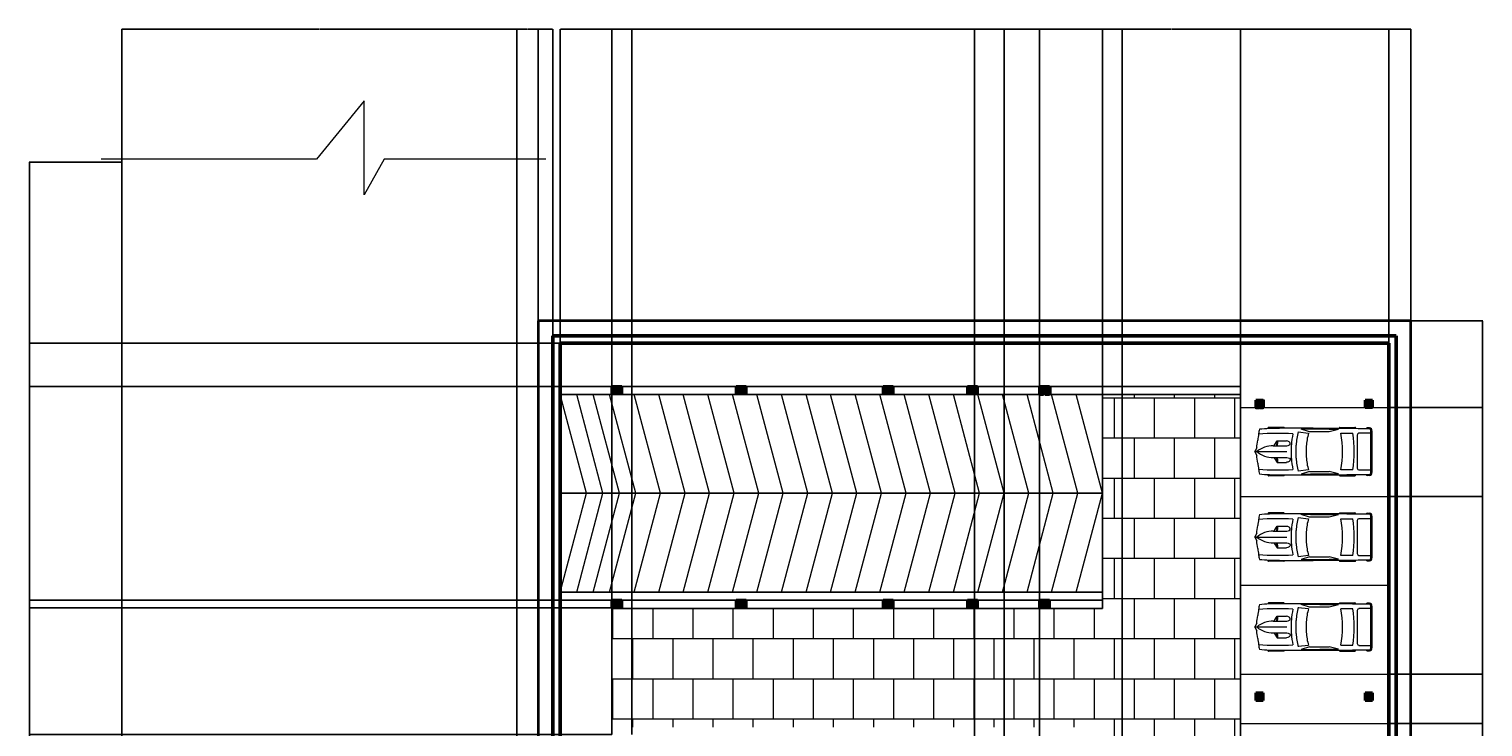
# Model space of a CAD drawing. Units: inches. Extents: x 154617 to 156384, y 250671 to 252576.
# Tile 6 of 6: x 154617 to 156384, y 251728 to 252576. Entities that reach past the tile are written whole.
import ezdxf

# ---------------------------------------------------------------- set-up
doc = ezdxf.new("R2010")
doc.units = ezdxf.units.IN
for name, color, linetype, lineweight in [('A-ANNO-DIMS', 2, 'Continuous', 18), ('A-EQPM-VEHI', 9, 'Continuous', 13), ('A-FLOR-DRIV', 5, 'Continuous', 25), ('A-FLOR-PATT', 112, 'Continuous', 13), ('A-FLOR-PRKG', 4, 'Continuous', 18), ('A-FLOR-RAMP', 7, 'Continuous', 25), ('A-FLOR-RAMP-PATT', 9, 'Continuous', 13), ('C-ANNO-BRKL', 7, 'Continuous', 18), ('C-PROP', 5, 'Continuous', 35), ('C-ROAD', 7, 'Continuous', 25), ('pillars', 6, 'Continuous', 40), ('walls', 4, 'Continuous', 50)]:
    doc.layers.add(name, color=color, linetype=linetype, lineweight=lineweight)
doc.styles.get("Standard").update_dxf_attribs({"font": 'arial.ttf'})
doc.dimstyles.get("Standard").update_dxf_attribs({"dimtxt": 0.18, "dimasz": 0.18, "dimexe": 0.18, "dimexo": 0.0625, "dimgap": 0.09, "dimtad": 0, "dimtih": 1, "dimtoh": 1, "dimdec": 4, "dimzin": 0, "dimdsep": 46, "dimtxsty": 'Standard', "dimcen": 0.09, "dimadec": 0, "dimazin": 0, "dimtfac": 1, "dimtdec": 4, "dimtofl": 0, "dimtmove": 0, "dimatfit": 3, "dimfxl": 1, "dimtolj": 1, "dimtzin": 0, "dimarcsym": 0})

# ---------------------------------------------------------------- blocks, each defined once
blk = doc.blocks.new('*U2')
for p, q in [((21.1, 37.4), (21.1, 36.8)), ((46.6, 38.9), (22.4, 38.9)), ((47.8, 37.4), (47.8, 37.4)), ((70, 31.5), (86.4, 29.4)), ((88, 31.9), (74.8, 35.9)), ((134.3, 35.6), (119.3, 31.8)), ((135.5, 37.1), (135.5, 37.4)), ((136.7, 38.9), (160.9, 38.9)), ((138.4, 29.4), (157.2, 29.4)), ((162.1, 37.4), (162.1, 36.8)), ((164.5, 26.4), (164.5, -26.4)), ((186.5, 29.4), (167, 29.4)), ((186.5, -33.5), (186.5, 33.5)), ((188.4, -32.8), (188.4, 32.8)), ((3.3, 6.1), (0.1, 0.4)), ((29.8, 9.5), (51.7, 9.5)), ((32.1, 9.5), (32.1, 11.2)), ((32.3, 11.6), (36.1, 17.2)), ((36.1, 17.2), (50.9, 17.2)), ((58.9, -10.8), (58.9, 10.8)), ((66.6, -10.5), (66.6, 10.5)), ((82.7, 8.5), (82.7, -8.5)), ((186.5, -10.5), (186.5, 10.5)), ((0, 0), (51.7, 0)), ((0.1, -0.4), (3.3, -6.1)), ((29.8, -9.5), (51.7, -9.5)), ((32.1, -9.5), (32.1, -11.2)), ((32.3, -11.6), (36.1, -17.2)), ((36.1, -17.2), (50.9, -17.2)), ((21.1, -37.4), (21.1, -36.8)), ((46.6, -38.9), (22.4, -38.9)), ((47.8, -37.4), (47.8, -37.4)), ((86.4, -29.4), (70, -31.5)), ((88, -31.9), (74.8, -35.9)), ((134.3, -35.6), (119.3, -31.8)), ((135.5, -37.1), (135.5, -37.4)), ((136.7, -38.9), (160.9, -38.9)), ((157.2, -29.4), (138.4, -29.4)), ((162.1, -37.4), (162.1, -36.8)), ((167, -29.4), (186.5, -29.4))]:
    blk.add_line(p, q)
for centre, major_axis, ratio, start_param, end_param in [((259.2, -27.5), (0, -305.3), 0.842304, 4.528606, 4.561838), ((266, -27.5), (0, 313.3), 0.842304, 1.367076, 1.39176), ((37.5, -594), (0, -623.3), 0.842304, 3.096046, 3.200911), ((41.2, -490.9), (0, 528.2), 0.842304, 0.00281, 0.075598), ((22.4, 37.4), (0, -1.48), 0.842304, 3.141593, 4.712389), ((64.5, -10555.6), (0, 10593), 0.842304, -0.013397, 0.002797), ((46.6, 37.4), (0, 1.48), 0.842304, -1.570796, 0), ((134.4, 5.4), (0, -89.8), 0.842304, 4.449482, 4.652344), ((135.3, 5.4), (0, 81.8), 0.842304, 1.245306, 1.50788), ((64.5, -10555.6), (0, -10591.5), 0.842304, 3.133765, 3.140441), ((149.6, 2.8), (0, -79.6), 0.842304, 4.372215, 4.640744), ((95.8, -3666.4), (0, -3698.2), 0.842304, 3.134049, 3.144098), ((136.7, 37.4), (0, -1.48), 0.842304, 3.141593, 4.712389), ((17.1, 0), (0, 147), 0.842304, 4.511394, 4.913384), ((35.9, 0), (0, 147), 0.842304, 4.511394, 4.913384), ((160.9, 37.4), (0, 1.48), 0.842304, -1.570796, 0), ((167, 26.4), (0, 2.96), 0.842304, 0, 1.570796), ((180.6, 35.8), (0, 2.22), 0.842304, -0.013017, 1.249894), ((64.5, -10556.4), (0, 10595.3), 0.842304, -0.013397, -0.013017), ((184, 32.8), (0, -5.25), 0.842304, 1.570796, 3.128196), ((184, 33.5), (0, -2.96), 0.842304, 1.570796, 3.128196), ((0.6, 0), (0, -0.74), 0.842304, 4.131459, 5.293319), ((-204.5, 52.4), (0, -251), 0.842304, 1.385369, 1.434372), ((29.8, -46.7), (0, 56.2), 0.842304, 0, 0.590319), ((32.7, 11.2), (0, 0.74), 0.842304, 0.879714, 1.570796), ((13, 17), (0, 27.4), 0.842304, 4.435146, 4.718221), ((14.2, 17), (0, 27.4), 0.842304, 4.435146, 4.718221), ((50.8, 13.3), (6.34, -0.36), 0.603834, -1.395552, 1.581315), ((-204.5, -52.4), (0, 251), 0.842304, -1.434372, -1.385369), ((29.8, 46.7), (0, 56.2), 0.842304, 2.551274, 3.141593), ((259.2, 27.5), (0, 305.3), 0.842304, 1.721348, 1.754579), ((32.7, -11.2), (0, -0.74), 0.842304, 4.712389, 5.403472), ((13, -17), (0, -27.4), 0.842304, 1.564964, 1.848039), ((14.2, -17), (0, -27.4), 0.842304, 1.564964, 1.848039), ((134.4, -5.4), (0, -89.8), 0.842304, -1.510751, -1.307889), ((135.3, -5.4), (0, -81.8), 0.842304, -1.50788, -1.245306), ((149.6, -2.8), (0, -79.6), 0.842304, -1.499151, -1.230623), ((266, 27.5), (0, 313.3), 0.842304, 1.749832, 1.774517), ((37.5, 594), (0, -623.3), 0.842304, -0.059319, 0.045547), ((41.2, 490.9), (0, -528.2), 0.842304, -0.075598, -0.00281), ((22.4, -37.4), (0, 1.48), 0.842304, 1.570796, 3.141593), ((64.5, 10555.6), (0, 10593), 0.842304, 3.138796, 3.15499), ((46.6, -37.4), (0, -1.48), 0.842304, 0, 1.570796), ((64.5, 10555.6), (0, -10591.5), 0.842304, 0.001152, 0.007828), ((95.8, 3666.4), (0, -3698.2), 0.842304, -0.002505, 0.007544), ((136.7, -37.4), (0, -1.48), 0.842304, -1.570796, 0), ((160.9, -37.4), (0, 1.48), 0.842304, 3.141593, 4.712389), ((167, -26.4), (0, -2.96), 0.842304, 4.712389, 6.283185), ((180.6, -35.8), (0, -2.22), 0.842304, -1.249894, 0.013017), ((64.5, 10556.4), (0, 10595.3), 0.842304, 3.15461, 3.15499), ((184, -32.8), (0, -5.25), 0.842304, 0.013397, 1.570796), ((184, -33.5), (0, 2.96), 0.842304, 3.15499, 4.712389)]:
    blk.add_ellipse(centre, major_axis=major_axis, ratio=ratio, start_param=start_param, end_param=end_param)
at = {"extrusion": (0, 0, -1)}
blk.add_ellipse((50.8, -13.3), major_axis=(6.34, 0.36), ratio=0.603834, start_param=-1.395552, end_param=1.581315, dxfattribs=at)
blk = doc.blocks.new('COL-RECT-12x9')
h = blk.add_hatch(color=256)
h.dxf.hatch_style = 1
h.paths.add_polyline_path([(12, 0), (12, 9), (0, 9), (0, 0)])
for p, q in [((12, 9), (0, 9)), ((0, 9), (0, 0)), ((12, 0), (12, 9)), ((0, 0), (12, 0))]:
    blk.add_line(p, q)
blk = doc.blocks.new('COL-RECT-9x9')
h = blk.add_hatch(color=256)
h.dxf.hatch_style = 1
h.paths.add_polyline_path([(0, 9.1), (0, 0), (9, 0), (9, 9.1)])
for p, q in [((9, 9.1), (0, 9.1)), ((0, 9.1), (0, 0)), ((0, 0), (9, 0)), ((9, 0), (9, 9.1))]:
    blk.add_line(p, q)
blk = doc.blocks.new('ROAD-BREAK')
for p, q in [((319.9, 114.2), (261.9, 43.3)), ((319.9, 0), (319.9, 114.2)), ((261.9, 43.3), (0, 43.3)), ((344.2, 43.3), (319.9, 0)), ((540.4, 43.3), (344.2, 43.3))]:
    blk.add_line(p, q)
blk = doc.blocks.new('*D9')
at = {"layer": 'A-ANNO-DIMS', "color": 0, "lineweight": -2, "transparency": 16777216}
for p, q in [((155844.6, 252133), (155844.6, 252131)), ((155844.8, 252131.2), (155849.5, 252131.2)), ((155856.4, 252131.2), (155851.7, 252131.2)), ((155856.6, 252133), (155856.6, 252131))]:
    blk.add_line(p, q, dxfattribs=at)
at = {"layer": 'A-ANNO-DIMS', "color": 0, "transparency": 16777216}
for points in [[(155844.8, 252131.3), (155844.8, 252131.2), (155844.6, 252131.2)], [(155856.4, 252131.3), (155856.4, 252131.2), (155856.6, 252131.2)]]:
    blk.add_solid(points, dxfattribs=at)
at = {"layer": 'Defpoints', "color": 0, "transparency": 16777216}
for p in [(155844.6, 252133), (155856.6, 252133), (155856.6, 252131.2)]:
    blk.add_point(p, dxfattribs=at)
at = {"layer": 'A-ANNO-DIMS', "color": 0, "transparency": 16777216, "insert": (155850.6, 252131.2), "char_height": 0.18, "attachment_point": 5}
blk.add_mtext('\\A1;COLUMN 12 TYP.', dxfattribs=at)
blk = doc.blocks.new('*D10')
at = {"layer": 'A-ANNO-DIMS', "color": 0, "lineweight": -2, "transparency": 16777216}
for p, q in [((155856.7, 252142), (155858.6, 252142)), ((155858.4, 252141.8), (155858.4, 252137.7)), ((155856.7, 252133), (155858.6, 252133)), ((155858.4, 252133.2), (155858.4, 252137.3))]:
    blk.add_line(p, q, dxfattribs=at)
at = {"layer": 'A-ANNO-DIMS', "color": 0, "transparency": 16777216}
for points in [[(155858.4, 252141.8), (155858.4, 252141.8), (155858.4, 252142)], [(155858.4, 252133.2), (155858.4, 252133.2), (155858.4, 252133)]]:
    blk.add_solid(points, dxfattribs=at)
at = {"layer": 'Defpoints', "color": 0, "transparency": 16777216}
for p in [(155856.6, 252142), (155858.4, 252142), (155856.6, 252133)]:
    blk.add_point(p, dxfattribs=at)
at = {"layer": 'A-ANNO-DIMS', "color": 0, "transparency": 16777216, "insert": (155858.4, 252137.5), "char_height": 0.18, "attachment_point": 5}
blk.add_mtext('\\A1;9 TYP.', dxfattribs=at)
blk = doc.blocks.new('*D11')
at = {"layer": 'A-ANNO-DIMS', "color": 0, "lineweight": -2, "transparency": 16777216}
for p, q in [((156116.5, 252125.4), (156118, 252125.4)), ((156117.8, 252125.2), (156117.8, 252121)), ((156117.8, 252116.5), (156117.8, 252120.7)), ((156116.5, 252116.3), (156118, 252116.3))]:
    blk.add_line(p, q, dxfattribs=at)
at = {"layer": 'A-ANNO-DIMS', "color": 0, "transparency": 16777216}
for points in [[(156117.8, 252125.2), (156117.9, 252125.2), (156117.8, 252125.4)], [(156117.8, 252116.5), (156117.9, 252116.5), (156117.8, 252116.3)]]:
    blk.add_solid(points, dxfattribs=at)
at = {"layer": 'Defpoints', "color": 0, "transparency": 16777216}
for p in [(156116.5, 252125.4), (156116.5, 252116.3), (156117.8, 252116.3)]:
    blk.add_point(p, dxfattribs=at)
at = {"layer": 'A-ANNO-DIMS', "color": 0, "transparency": 16777216, "insert": (156117.8, 252120.8), "char_height": 0.18, "attachment_point": 5}
blk.add_mtext('\\A1;COLUMN 9 TYP.', dxfattribs=at)
blk = doc.blocks.new('*D12')
at = {"layer": 'A-ANNO-DIMS', "color": 0, "lineweight": -2, "transparency": 16777216}
for p, q in [((156107.5, 252116.2), (156107.5, 252114.8)), ((156107.7, 252114.9), (156111.5, 252114.9)), ((156116.3, 252114.9), (156112.4, 252114.9)), ((156116.5, 252116.2), (156116.5, 252114.8))]:
    blk.add_line(p, q, dxfattribs=at)
at = {"layer": 'A-ANNO-DIMS', "color": 0, "transparency": 16777216}
for points in [[(156107.7, 252115), (156107.7, 252114.9), (156107.5, 252114.9)], [(156116.3, 252115), (156116.3, 252114.9), (156116.5, 252114.9)]]:
    blk.add_solid(points, dxfattribs=at)
at = {"layer": 'Defpoints', "color": 0, "transparency": 16777216}
for p in [(156107.5, 252116.3), (156107.5, 252114.9), (156116.5, 252116.3)]:
    blk.add_point(p, dxfattribs=at)
at = {"layer": 'A-ANNO-DIMS', "color": 0, "transparency": 16777216, "insert": (156112, 252114.9), "char_height": 0.18, "attachment_point": 5}
blk.add_mtext('\\A1;9 TYP.', dxfattribs=at)
blk = doc.blocks.new('*D20')
at = {"layer": 'A-ANNO-DIMS', "color": 0, "lineweight": -2, "transparency": 16777216}
for p, q in [((156296.2, 252221.5), (156383.4, 252221.5)), ((156383.2, 252221.3), (156383.2, 251628.5)), ((156383.2, 251035.2), (156383.2, 251628.1)), ((156296.2, 251035), (156383.4, 251035))]:
    blk.add_line(p, q, dxfattribs=at)
at = {"layer": 'A-ANNO-DIMS', "color": 0, "transparency": 16777216}
for points in [[(156383.2, 252221.3), (156383.2, 252221.3), (156383.2, 252221.5)], [(156383.2, 251035.2), (156383.2, 251035.2), (156383.2, 251035)]]:
    blk.add_solid(points, dxfattribs=at)
at = {"layer": 'Defpoints', "color": 0, "transparency": 16777216}
for p in [(156296.1, 252221.5), (156383.2, 252221.5), (156296.1, 251035)]:
    blk.add_point(p, dxfattribs=at)
at = {"layer": 'A-ANNO-DIMS', "color": 0, "transparency": 16777216, "insert": (156383.2, 251628.3), "char_height": 0.18, "attachment_point": 5}
blk.add_mtext('\\A1;1186.5', dxfattribs=at)
blk = doc.blocks.new('*D21')
at = {"layer": 'A-ANNO-DIMS', "color": 0, "lineweight": -2, "transparency": 16777216}
for p, q in [((154729.2, 252414.6), (154729.2, 252576.2)), ((154729.4, 252576), (154968.9, 252576)), ((155209.1, 252576), (154969.5, 252576)), ((155209.2, 252414.6), (155209.2, 252576.2))]:
    blk.add_line(p, q, dxfattribs=at)
at = {"layer": 'A-ANNO-DIMS', "color": 0, "transparency": 16777216}
for points in [[(154729.4, 252576), (154729.4, 252576), (154729.2, 252576)], [(155209.1, 252576), (155209.1, 252576), (155209.2, 252576)]]:
    blk.add_solid(points, dxfattribs=at)
at = {"layer": 'Defpoints', "color": 0, "transparency": 16777216}
for p in [(155209.2, 252576), (154729.2, 252414.5), (155209.2, 252414.5)]:
    blk.add_point(p, dxfattribs=at)
at = {"layer": 'A-ANNO-DIMS', "color": 0, "transparency": 16777216, "insert": (154969.2, 252576), "char_height": 0.18, "attachment_point": 5}
blk.add_mtext('\\A1;480', dxfattribs=at)
blk = doc.blocks.new('*D22')
at = {"layer": 'A-ANNO-DIMS', "color": 0, "lineweight": -2, "transparency": 16777216}
for p, q in [((155209.2, 252414.6), (155209.2, 252576.2)), ((155209.4, 252576), (155221.8, 252576)), ((155234.9, 252576), (155222.6, 252576)), ((155235.1, 252221.6), (155235.1, 252576.2))]:
    blk.add_line(p, q, dxfattribs=at)
at = {"layer": 'A-ANNO-DIMS', "color": 0, "transparency": 16777216}
for points in [[(155209.4, 252576), (155209.4, 252576), (155209.2, 252576)], [(155234.9, 252576), (155234.9, 252576), (155235.1, 252576)]]:
    blk.add_solid(points, dxfattribs=at)
at = {"layer": 'Defpoints', "color": 0, "transparency": 16777216}
for p in [(155235.1, 252576), (155209.2, 252414.5), (155235.1, 252221.5)]:
    blk.add_point(p, dxfattribs=at)
at = {"layer": 'A-ANNO-DIMS', "color": 0, "transparency": 16777216, "insert": (155222.2, 252576), "char_height": 0.18, "attachment_point": 5}
blk.add_mtext('\\A1;25.86', dxfattribs=at)
blk = doc.blocks.new('*D23')
at = {"layer": 'A-ANNO-DIMS', "color": 0, "lineweight": -2, "transparency": 16777216}
for p, q in [((154729.2, 252414.5), (154616.7, 252414.5)), ((154616.9, 252414.3), (154616.9, 251606.6)), ((154616.9, 250798.4), (154616.9, 251606.2)), ((154729.2, 250798.3), (154616.7, 250798.3))]:
    blk.add_line(p, q, dxfattribs=at)
at = {"layer": 'A-ANNO-DIMS', "color": 0, "transparency": 16777216}
for points in [[(154616.9, 252414.3), (154616.9, 252414.3), (154616.9, 252414.5)], [(154616.9, 250798.4), (154616.9, 250798.4), (154616.9, 250798.3)]]:
    blk.add_solid(points, dxfattribs=at)
at = {"layer": 'Defpoints', "color": 0, "transparency": 16777216}
for p in [(154616.9, 252414.5), (154729.2, 252414.5), (154729.2, 250798.3)]:
    blk.add_point(p, dxfattribs=at)
at = {"layer": 'A-ANNO-DIMS', "color": 0, "transparency": 16777216, "insert": (154616.9, 251606.4), "char_height": 0.18, "attachment_point": 5}
blk.add_mtext('\\A1;1616.2', dxfattribs=at)
blk = doc.blocks.new('*D25')
at = {"layer": 'A-ANNO-DIMS', "color": 0, "lineweight": -2, "transparency": 16777216}
for p, q in [((155262.1, 252142.1), (155262.1, 252576.2)), ((155262.3, 252576), (155591.3, 252576)), ((155920.9, 252576), (155591.9, 252576)), ((155921.1, 252142.1), (155921.1, 252576.2))]:
    blk.add_line(p, q, dxfattribs=at)
at = {"layer": 'A-ANNO-DIMS', "color": 0, "transparency": 16777216}
for points in [[(155262.3, 252576), (155262.3, 252576), (155262.1, 252576)], [(155920.9, 252576), (155920.9, 252576), (155921.1, 252576)]]:
    blk.add_solid(points, dxfattribs=at)
at = {"layer": 'Defpoints', "color": 0, "transparency": 16777216}
for p in [(155921.1, 252576), (155262.1, 252142), (155921.1, 252142)]:
    blk.add_point(p, dxfattribs=at)
at = {"layer": 'A-ANNO-DIMS', "color": 0, "transparency": 16777216, "insert": (155591.6, 252576), "char_height": 0.18, "attachment_point": 5}
blk.add_mtext('\\A1;659', dxfattribs=at)
blk = doc.blocks.new('*D26')
at = {"layer": 'A-ANNO-DIMS', "color": 0, "lineweight": -2, "transparency": 16777216}
for p, q in [((155921.1, 252142.1), (155921.1, 252576.2)), ((155921.3, 252576), (156004.8, 252576)), ((156088.9, 252576), (156005.4, 252576)), ((156089.1, 252142.1), (156089.1, 252576.2))]:
    blk.add_line(p, q, dxfattribs=at)
at = {"layer": 'A-ANNO-DIMS', "color": 0, "transparency": 16777216}
for points in [[(155921.3, 252576), (155921.3, 252576), (155921.1, 252576)], [(156088.9, 252576), (156088.9, 252576), (156089.1, 252576)]]:
    blk.add_solid(points, dxfattribs=at)
at = {"layer": 'Defpoints', "color": 0, "transparency": 16777216}
for p in [(156089.1, 252576), (155921.1, 252142), (156089.1, 252142)]:
    blk.add_point(p, dxfattribs=at)
at = {"layer": 'A-ANNO-DIMS', "color": 0, "transparency": 16777216, "insert": (156005.1, 252576), "char_height": 0.18, "attachment_point": 5}
blk.add_mtext('\\A1;168', dxfattribs=at)
blk = doc.blocks.new('*D27')
at = {"layer": 'A-ANNO-DIMS', "color": 0, "lineweight": -2, "transparency": 16777216}
for p, q in [((156089.1, 252116.4), (156089.1, 252576.2)), ((156089.3, 252576), (156178.8, 252576)), ((156268.9, 252576), (156179.4, 252576)), ((156269.1, 252116.4), (156269.1, 252576.2))]:
    blk.add_line(p, q, dxfattribs=at)
at = {"layer": 'A-ANNO-DIMS', "color": 0, "transparency": 16777216}
for points in [[(156089.3, 252576), (156089.3, 252576), (156089.1, 252576)], [(156268.9, 252576), (156268.9, 252576), (156269.1, 252576)]]:
    blk.add_solid(points, dxfattribs=at)
at = {"layer": 'Defpoints', "color": 0, "transparency": 16777216}
for p in [(156269.1, 252576), (156089.1, 252116.3), (156269.1, 252116.3)]:
    blk.add_point(p, dxfattribs=at)
at = {"layer": 'A-ANNO-DIMS', "color": 0, "transparency": 16777216, "insert": (156179.1, 252576), "char_height": 0.18, "attachment_point": 5}
blk.add_mtext('\\A1;180', dxfattribs=at)
blk = doc.blocks.new('*D28')
at = {"layer": 'A-ANNO-DIMS', "color": 0, "lineweight": -2, "transparency": 16777216}
for p, q in [((155262, 252194.5), (154616.7, 252194.5)), ((154616.9, 252194.3), (154616.9, 252168.5)), ((154616.9, 252142.2), (154616.9, 252168.1)), ((155262, 252142), (154616.7, 252142))]:
    blk.add_line(p, q, dxfattribs=at)
at = {"layer": 'A-ANNO-DIMS', "color": 0, "transparency": 16777216}
for points in [[(154616.9, 252194.3), (154616.9, 252194.3), (154616.9, 252194.5)], [(154616.9, 252142.2), (154616.9, 252142.2), (154616.9, 252142)]]:
    blk.add_solid(points, dxfattribs=at)
at = {"layer": 'Defpoints', "color": 0, "transparency": 16777216}
for p in [(154616.9, 252194.5), (155262.1, 252194.5), (155262.1, 252142)]:
    blk.add_point(p, dxfattribs=at)
at = {"layer": 'A-ANNO-DIMS', "color": 0, "transparency": 16777216, "insert": (154616.9, 252168.3), "char_height": 0.18, "attachment_point": 5}
blk.add_mtext('\\A1;52.5', dxfattribs=at)
blk = doc.blocks.new('*D29')
at = {"layer": 'A-ANNO-DIMS', "color": 0, "lineweight": -2, "transparency": 16777216}
for p, q in [((155262, 252142), (154616.7, 252142)), ((154616.9, 252141.8), (154616.9, 252012.2)), ((154616.9, 251882.2), (154616.9, 252011.8)), ((155262, 251882), (154616.7, 251882))]:
    blk.add_line(p, q, dxfattribs=at)
at = {"layer": 'A-ANNO-DIMS', "color": 0, "transparency": 16777216}
for points in [[(154616.9, 252141.8), (154616.9, 252141.8), (154616.9, 252142)], [(154616.9, 251882.2), (154616.9, 251882.2), (154616.9, 251882)]]:
    blk.add_solid(points, dxfattribs=at)
at = {"layer": 'Defpoints', "color": 0, "transparency": 16777216}
for p in [(154616.9, 252142), (155262.1, 252142), (155262.1, 251882)]:
    blk.add_point(p, dxfattribs=at)
at = {"layer": 'A-ANNO-DIMS', "color": 0, "transparency": 16777216, "insert": (154616.9, 252012), "char_height": 0.18, "attachment_point": 5}
blk.add_mtext('\\A1;260', dxfattribs=at)
blk = doc.blocks.new('*D32')
at = {"layer": 'A-ANNO-DIMS', "color": 0, "lineweight": -2, "transparency": 16777216}
for p, q in [((155324.8, 251873), (154616.7, 251873)), ((154616.9, 251872.8), (154616.9, 251796.2)), ((154616.9, 251719.2), (154616.9, 251795.8)), ((155324.8, 251719), (154616.7, 251719))]:
    blk.add_line(p, q, dxfattribs=at)
at = {"layer": 'A-ANNO-DIMS', "color": 0, "transparency": 16777216}
for points in [[(154616.9, 251872.8), (154616.9, 251872.8), (154616.9, 251873)], [(154616.9, 251719.2), (154616.9, 251719.2), (154616.9, 251719)]]:
    blk.add_solid(points, dxfattribs=at)
at = {"layer": 'Defpoints', "color": 0, "transparency": 16777216}
for p in [(154616.9, 251873), (155324.8, 251873), (155324.8, 251719)]:
    blk.add_point(p, dxfattribs=at)
at = {"layer": 'A-ANNO-DIMS', "color": 0, "transparency": 16777216, "insert": (154616.9, 251796), "char_height": 0.18, "attachment_point": 5}
blk.add_mtext('\\A1;154', dxfattribs=at)
blk = doc.blocks.new('*D41')
at = {"layer": 'A-ANNO-DIMS', "color": 0, "lineweight": -2, "transparency": 16777216}
for p, q in [((156269.2, 252116.3), (156383.4, 252116.3)), ((156383.2, 252116.1), (156383.2, 252062.5)), ((156383.2, 252008.5), (156383.2, 252062.1)), ((156269.2, 252008.3), (156383.4, 252008.3))]:
    blk.add_line(p, q, dxfattribs=at)
at = {"layer": 'A-ANNO-DIMS', "color": 0, "transparency": 16777216}
for points in [[(156383.2, 252116.1), (156383.2, 252116.1), (156383.2, 252116.3)], [(156383.2, 252008.5), (156383.2, 252008.5), (156383.2, 252008.3)]]:
    blk.add_solid(points, dxfattribs=at)
at = {"layer": 'Defpoints', "color": 0, "transparency": 16777216}
for p in [(156269.1, 252116.3), (156383.2, 252116.3), (156269.1, 252008.3)]:
    blk.add_point(p, dxfattribs=at)
at = {"layer": 'A-ANNO-DIMS', "color": 0, "transparency": 16777216, "insert": (156383.2, 252062.3), "char_height": 0.18, "attachment_point": 5}
blk.add_mtext('\\A1;108', dxfattribs=at)
blk = doc.blocks.new('*D42')
at = {"layer": 'A-ANNO-DIMS', "color": 0, "lineweight": -2, "transparency": 16777216}
for p, q in [((156269.2, 252008.3), (156383.4, 252008.3)), ((156383.2, 252008.1), (156383.2, 251900.5)), ((156383.2, 251792.5), (156383.2, 251900.1)), ((156269.2, 251792.3), (156383.4, 251792.3))]:
    blk.add_line(p, q, dxfattribs=at)
at = {"layer": 'A-ANNO-DIMS', "color": 0, "transparency": 16777216}
for points in [[(156383.2, 252008.1), (156383.2, 252008.1), (156383.2, 252008.3)], [(156383.2, 251792.5), (156383.2, 251792.5), (156383.2, 251792.3)]]:
    blk.add_solid(points, dxfattribs=at)
at = {"layer": 'Defpoints', "color": 0, "transparency": 16777216}
for p in [(156269.1, 252008.3), (156383.2, 252008.3), (156269.1, 251792.3)]:
    blk.add_point(p, dxfattribs=at)
at = {"layer": 'A-ANNO-DIMS', "color": 0, "transparency": 16777216, "insert": (156383.2, 251900.3), "char_height": 0.18, "attachment_point": 5}
blk.add_mtext('\\A1;216', dxfattribs=at)
blk = doc.blocks.new('*D43')
at = {"layer": 'A-ANNO-DIMS', "color": 0, "lineweight": -2, "transparency": 16777216}
for p, q in [((156269.2, 251792.3), (156383.4, 251792.3)), ((156383.2, 251792.1), (156383.2, 251762.5)), ((156383.2, 251732.5), (156383.2, 251762.1)), ((156269.2, 251732.3), (156383.4, 251732.3))]:
    blk.add_line(p, q, dxfattribs=at)
at = {"layer": 'A-ANNO-DIMS', "color": 0, "transparency": 16777216}
for points in [[(156383.2, 251792.1), (156383.2, 251792.1), (156383.2, 251792.3)], [(156383.2, 251732.5), (156383.2, 251732.5), (156383.2, 251732.3)]]:
    blk.add_solid(points, dxfattribs=at)
at = {"layer": 'Defpoints', "color": 0, "transparency": 16777216}
for p in [(156269.1, 251792.3), (156383.2, 251792.3), (156269.1, 251732.3)]:
    blk.add_point(p, dxfattribs=at)
at = {"layer": 'A-ANNO-DIMS', "color": 0, "transparency": 16777216, "insert": (156383.2, 251762.3), "char_height": 0.18, "attachment_point": 5}
blk.add_mtext('\\A1;60', dxfattribs=at)
blk = doc.blocks.new('*D44')
at = {"layer": 'A-ANNO-DIMS', "color": 0, "lineweight": -2, "transparency": 16777216}
for p, q in [((156269.2, 251732.3), (156383.4, 251732.3)), ((156383.2, 251732.1), (156383.2, 251678.5)), ((156383.2, 251624.5), (156383.2, 251678.1)), ((156269.2, 251624.3), (156383.4, 251624.3))]:
    blk.add_line(p, q, dxfattribs=at)
at = {"layer": 'A-ANNO-DIMS', "color": 0, "transparency": 16777216}
for points in [[(156383.2, 251732.1), (156383.2, 251732.1), (156383.2, 251732.3)], [(156383.2, 251624.5), (156383.2, 251624.5), (156383.2, 251624.3)]]:
    blk.add_solid(points, dxfattribs=at)
at = {"layer": 'Defpoints', "color": 0, "transparency": 16777216}
for p in [(156269.1, 251732.3), (156383.2, 251732.3), (156269.1, 251624.3)]:
    blk.add_point(p, dxfattribs=at)
at = {"layer": 'A-ANNO-DIMS', "color": 0, "transparency": 16777216, "insert": (156383.2, 251678.3), "char_height": 0.18, "attachment_point": 5}
blk.add_mtext('\\A1;108', dxfattribs=at)
blk = doc.blocks.new('*D58')
at = {"layer": 'A-ANNO-DIMS', "color": 0, "lineweight": -2, "transparency": 16777216}
for p, q in [((155844.6, 251299.6), (155844.6, 252576.2)), ((155844.8, 252576), (155894.5, 252576)), ((155944.9, 252576), (155895.2, 252576)), ((155945.1, 251299.6), (155945.1, 252576.2))]:
    blk.add_line(p, q, dxfattribs=at)
at = {"layer": 'A-ANNO-DIMS', "color": 0, "transparency": 16777216}
for points in [[(155844.8, 252576), (155844.8, 252576), (155844.6, 252576)], [(155944.9, 252576), (155944.9, 252576), (155945.1, 252576)]]:
    blk.add_solid(points, dxfattribs=at)
at = {"layer": 'Defpoints', "color": 0, "transparency": 16777216}
for p in [(155945.1, 252576), (155844.6, 251299.5), (155945.1, 251299.5)]:
    blk.add_point(p, dxfattribs=at)
at = {"layer": 'A-ANNO-DIMS', "color": 0, "transparency": 16777216, "insert": (155894.8, 252576), "char_height": 0.18, "attachment_point": 5}
blk.add_mtext('\\A1;100.5', dxfattribs=at)
blk = doc.blocks.new('*D65')
at = {"layer": 'A-ANNO-DIMS', "color": 0, "lineweight": -2, "transparency": 16777216}
for p, q in [((156269.1, 252194.6), (156269.1, 252576.2)), ((156269.3, 252576), (156282.4, 252576)), ((156295.9, 252576), (156282.8, 252576)), ((156296.1, 252221.6), (156296.1, 252576.2))]:
    blk.add_line(p, q, dxfattribs=at)
at = {"layer": 'A-ANNO-DIMS', "color": 0, "transparency": 16777216}
for points in [[(156269.3, 252576), (156269.3, 252576), (156269.1, 252576)], [(156295.9, 252576), (156295.9, 252576), (156296.1, 252576)]]:
    blk.add_solid(points, dxfattribs=at)
at = {"layer": 'Defpoints', "color": 0, "transparency": 16777216}
for p in [(156296.1, 252576), (156296.1, 252221.5), (156269.1, 252194.5)]:
    blk.add_point(p, dxfattribs=at)
at = {"layer": 'A-ANNO-DIMS', "color": 0, "transparency": 16777216, "insert": (156282.6, 252576), "char_height": 0.18, "attachment_point": 5}
blk.add_mtext('\\A1;27', dxfattribs=at)
blk = doc.blocks.new('*D66')
at = {"layer": 'A-ANNO-DIMS', "color": 0, "lineweight": -2, "transparency": 16777216}
for p, q in [((155235.1, 252221.6), (155235.1, 252576.2)), ((155235.3, 252576), (155243.9, 252576)), ((155252.9, 252576), (155244.3, 252576)), ((155253.1, 252203.6), (155253.1, 252576.2))]:
    blk.add_line(p, q, dxfattribs=at)
at = {"layer": 'A-ANNO-DIMS', "color": 0, "transparency": 16777216}
for points in [[(155235.3, 252576), (155235.3, 252576), (155235.1, 252576)], [(155252.9, 252576), (155252.9, 252576), (155253.1, 252576)]]:
    blk.add_solid(points, dxfattribs=at)
at = {"layer": 'Defpoints', "color": 0, "transparency": 16777216}
for p in [(155253.1, 252576), (155235.1, 252221.5), (155253.1, 252203.5)]:
    blk.add_point(p, dxfattribs=at)
at = {"layer": 'A-ANNO-DIMS', "color": 0, "transparency": 16777216, "insert": (155244.1, 252576), "char_height": 0.18, "attachment_point": 5}
blk.add_mtext('\\A1;18', dxfattribs=at)
blk = doc.blocks.new('*D67')
at = {"layer": 'A-ANNO-DIMS', "color": 0, "lineweight": -2, "transparency": 16777216}
for p, q in [((155324.8, 251719.1), (155324.8, 252576.2)), ((155325, 252576), (155336.5, 252576)), ((155348.8, 252576), (155337.3, 252576)), ((155349, 251719.1), (155349, 252576.2))]:
    blk.add_line(p, q, dxfattribs=at)
at = {"layer": 'A-ANNO-DIMS', "color": 0, "transparency": 16777216}
for points in [[(155325, 252576), (155325, 252576), (155324.8, 252576)], [(155348.8, 252576), (155348.8, 252576), (155349, 252576)]]:
    blk.add_solid(points, dxfattribs=at)
at = {"layer": 'Defpoints', "color": 0, "transparency": 16777216}
for p in [(155349, 252576), (155324.8, 251719), (155349, 251719)]:
    blk.add_point(p, dxfattribs=at)
at = {"layer": 'A-ANNO-DIMS', "color": 0, "transparency": 16777216, "insert": (155336.9, 252576), "char_height": 0.18, "attachment_point": 5}
blk.add_mtext('\\A1;24.14', dxfattribs=at)
blk = doc.blocks.new('*D70')
at = {"layer": 'A-ANNO-DIMS', "color": 0, "lineweight": -2, "transparency": 16777216}
for p, q in [((155765.6, 251299.6), (155765.6, 252576.2)), ((155765.8, 252576), (155783.4, 252576)), ((155801.4, 252576), (155783.8, 252576)), ((155801.6, 251299.6), (155801.6, 252576.2))]:
    blk.add_line(p, q, dxfattribs=at)
at = {"layer": 'A-ANNO-DIMS', "color": 0, "transparency": 16777216}
for points in [[(155765.8, 252576), (155765.8, 252576), (155765.6, 252576)], [(155801.4, 252576), (155801.4, 252576), (155801.6, 252576)]]:
    blk.add_solid(points, dxfattribs=at)
at = {"layer": 'Defpoints', "color": 0, "transparency": 16777216}
for p in [(155801.6, 252576), (155765.6, 251299.5), (155801.6, 251299.5)]:
    blk.add_point(p, dxfattribs=at)
at = {"layer": 'A-ANNO-DIMS', "color": 0, "transparency": 16777216, "insert": (155783.6, 252576), "char_height": 0.18, "attachment_point": 5}
blk.add_mtext('\\A1;36', dxfattribs=at)

msp = doc.modelspace()

# ---------------------------------------------------------------- hatches: boundary and pattern name
at = {"layer": 'A-FLOR-PATT'}
h = msp.add_hatch(dxfattribs=at)
h.set_pattern_fill('AR-B88', color=256, scale=0.24)
h.set_pattern_definition([(0, (0, -2.5), (0, 48.768), []), (90, (0, -2.5), (-24.384, 48.768), [48.768, -48.768])])
h.paths.add_polyline_path([(155324.842, 251443.526), (155324.842, 251299.526), (155945.097, 251299.526), (155945.097, 251119.526), (156089.097, 251119.526), (156089.097, 252132.026), (155921.097, 252132.026), (155921.097, 251872.026), (155324.842, 251872.026), (155324.842, 251728.026), (155921.097, 251728.026), (155921.097, 251443.526)])
at = {"layer": 'A-FLOR-RAMP-PATT'}
h = msp.add_hatch(dxfattribs=at)
h.set_pattern_fill('ANSI31', color=256, scale=6.0867434, angle=59.923503, style=0)
h.paths.add_polyline_path([(155294.018, 252012.026), (155334.138, 252012.026), (155302.155, 252132.026), (155262.035, 252132.026)])
h = msp.add_hatch(dxfattribs=at)
h.set_pattern_fill('ANSI31', color=256, scale=9.08246, angle=59.92146, style=0)
h.paths.add_polyline_path([(155354.018, 252012.026), (155921.157, 252012.026), (155889.179, 252132.026), (155322.04, 252132.026)])
h = msp.add_hatch(dxfattribs=at)
h.set_pattern_fill('ANSI31', color=256, scale=6.0868147, angle=30.079012, style=0)
h.paths.add_polyline_path([(155262.037, 251892.026), (155302.157, 251892.026), (155334.134, 252012.026), (155294.014, 252012.026)])
h = msp.add_hatch(dxfattribs=at)
h.set_pattern_fill('ANSI31', color=256, scale=9.0823579, angle=30.076133, style=0)
h.paths.add_polyline_path([(155322.037, 251892.026), (155889.177, 251892.026), (155921.16, 252012.026), (155354.02, 252012.026)])

# ---------------------------------------------------------------- linework, layer by layer
at = {"layer": 'A-FLOR-DRIV'}
for p, q in [((156089.097, 251119.526), (156089.097, 252142.026)), ((155921.097, 251872.026), (155324.842, 251872.026)), ((155324.842, 251872.026), (155324.842, 251728.236))]:
    msp.add_line(p, q, dxfattribs=at)
at = {"layer": 'A-FLOR-PRKG'}
for p, q in [((156089.097, 252116.297), (156269.097, 252116.297)), ((156089.097, 252008.297), (156269.097, 252008.297)), ((156089.097, 251900.297), (156269.097, 251900.297)), ((156089.097, 251792.297), (156269.097, 251792.297)), ((156089.097, 251732.297), (156269.097, 251732.297))]:
    msp.add_line(p, q, dxfattribs=at)
at = {"layer": 'A-FLOR-RAMP'}
for p, q in [((156089.097, 252142.026), (155262.097, 252142.026)), ((155921.097, 251872.026), (155921.097, 252142.026)), ((156089.097, 252132.026), (155262.097, 252132.026)), ((155921.097, 252012.026), (155262.097, 252012.026)), ((155921.097, 251892.026), (155262.097, 251892.026)), ((155921.097, 251882.026), (155262.097, 251882.026))]:
    msp.add_line(p, q, dxfattribs=at)
at = {"layer": 'C-PROP'}
for p, q in [((155235.097, 252221.526), (155235.097, 251035.026)), ((156296.097, 252221.526), (155235.097, 252221.526)), ((156296.097, 251035.026), (156296.097, 252221.526))]:
    msp.add_line(p, q, dxfattribs=at)
at = {"layer": 'C-ROAD'}
for p, q in [((154729.237, 252414.495), (154729.237, 250798.266)), ((155209.237, 252414.495), (155209.237, 250798.266))]:
    msp.add_line(p, q, dxfattribs=at)
at = {"layer": 'walls'}
for p, q in [((156278.097, 252203.526), (155253.097, 252203.526)), ((155253.097, 252203.526), (155253.097, 251053.026)), ((156269.097, 252194.526), (155262.097, 252194.526)), ((155262.097, 252194.526), (155262.097, 251062.026)), ((156269.097, 251062.026), (156269.097, 252194.526)), ((156278.097, 251053.026), (156278.097, 252203.526))]:
    msp.add_line(p, q, dxfattribs=at)

# ---------------------------------------------------------------- block references
at = {"layer": 'A-EQPM-VEHI', "xscale": 0.7581398915747906, "yscale": 0.7581398915747906, "zscale": 0.7581398915747906}
for p in [(156106.107, 252062.684), (156106.107, 251958.873), (156106.107, 251849.558)]:
    msp.add_blockref('*U2', p, dxfattribs=at)
at = {"layer": 'C-ANNO-BRKL'}
msp.add_blockref('ROAD-BREAK', (154704.015, 252374.708), dxfattribs=at)
at = {"layer": 'pillars'}
for name, p in [('COL-RECT-12x9', (155324.841, 252133.027)), ('COL-RECT-12x9', (155475.979, 252133.027)), ('COL-RECT-12x9', (155654.613, 252133.027)), ('COL-RECT-12x9', (155757.202, 252133.027)), ('COL-RECT-12x9', (155844.597, 252133.027)), ('COL-RECT-9x9', (156240.355, 252116.297)), ('COL-RECT-12x9', (155324.841, 251873.027)), ('COL-RECT-12x9', (155475.979, 251873.027)), ('COL-RECT-12x9', (155654.613, 251873.027)), ('COL-RECT-12x9', (155757.202, 251873.027)), ('COL-RECT-12x9', (155844.597, 251873.027))]:
    msp.add_blockref(name, p, dxfattribs=at)
at = {"layer": 'pillars', "rotation": 180}
for p in [(156116.47, 252125.389), (156116.47, 251769.457), (156249.356, 251769.457)]:
    msp.add_blockref('COL-RECT-9x9', p, dxfattribs=at)

# ---------------------------------------------------------------- dimensions: what is measured, and where the dimension line sits
at = {"layer": 'A-ANNO-DIMS'}
for base, p1, p2, override, picture, middle in [((155209.237, 252575.997), (154729.237, 252414.495), (155209.237, 252414.495), {"dimdec": 0, "dimlfac": 1, "dimrnd": 0, "dimzin": 0, "dimdsep": 46, "dimlunit": 2}, '*D21', (154969.237, 252575.997)), ((155235.097, 252575.997), (155209.237, 252414.495), (155235.097, 252221.526), {"dimdec": 2, "dimlfac": 1, "dimrnd": 0, "dimzin": 0, "dimdsep": 46, "dimlunit": 2}, '*D22', (155222.167, 252575.997)), ((155253.097, 252575.997), (155235.097, 252221.526), (155253.097, 252203.526), {"dimdec": 0, "dimlfac": 1, "dimrnd": 0, "dimzin": 0, "dimdsep": 46, "dimlunit": 2}, '*D66', (155244.097, 252575.997)), ((155921.097, 252575.997), (155262.097, 252142.026), (155921.097, 252142.026), {"dimdec": 0, "dimlfac": 1, "dimrnd": 0, "dimzin": 0, "dimdsep": 46, "dimlunit": 2}, '*D25', (155591.597, 252575.997)), ((155348.982, 252575.997), (155324.842, 251719.026), (155348.982, 251719.026), {"dimdec": 2, "dimlfac": 1, "dimrnd": 0, "dimzin": 0, "dimdsep": 46, "dimlunit": 2}, '*D67', (155336.912, 252575.997)), ((155801.597, 252575.997), (155765.597, 251299.526), (155801.597, 251299.526), {"dimdec": 0, "dimlfac": 1, "dimrnd": 0, "dimzin": 0, "dimdsep": 46, "dimlunit": 2}, '*D70', (155783.597, 252575.997)), ((155945.097, 252575.997), (155844.597, 251299.526), (155945.097, 251299.526), {"dimdec": 1, "dimlfac": 1, "dimrnd": 0, "dimzin": 0, "dimdsep": 46, "dimlunit": 2}, '*D58', (155894.847, 252575.997)), ((156089.097, 252575.997), (155921.097, 252142.026), (156089.097, 252142.026), {"dimdec": 0, "dimlfac": 1, "dimrnd": 0, "dimzin": 0, "dimdsep": 46, "dimlunit": 2}, '*D26', (156005.097, 252575.997)), ((156269.097, 252575.997), (156089.097, 252116.297), (156269.097, 252116.297), {"dimdec": 0, "dimlfac": 1, "dimrnd": 0, "dimzin": 0, "dimdsep": 46, "dimlunit": 2}, '*D27', (156179.097, 252575.997)), ((156296.097, 252575.997), (156269.097, 252194.526), (156296.097, 252221.526), {"dimdec": 0, "dimlfac": 1, "dimrnd": 0, "dimzin": 0, "dimdsep": 46, "dimlunit": 2}, '*D65', (156282.597, 252575.997))]:
    dim = msp.add_linear_dim(base=base, p1=p1, p2=p2, dimstyle='Standard', override=override, dxfattribs=at)
    dim.commit()
    dim.dimension.update_dxf_attribs({"geometry": picture, "text_midpoint": middle})
for base, p1, p2, override, picture, middle in [((154616.915, 252414.495), (154729.237, 250798.266), (154729.237, 252414.495), {"dimdec": 1, "dimlfac": 1, "dimrnd": 0, "dimzin": 0, "dimdsep": 46, "dimlunit": 2}, '*D23', (154616.915, 251606.381)), ((156383.197, 252221.526), (156296.097, 251035.026), (156296.097, 252221.526), {"dimdec": 1, "dimlfac": 1, "dimrnd": 0, "dimzin": 0, "dimdsep": 46, "dimlunit": 2}, '*D20', (156383.197, 251628.276)), ((154616.915, 252194.526), (155262.097, 252142.026), (155262.097, 252194.526), {"dimdec": 1, "dimlfac": 1, "dimrnd": 0, "dimzin": 0, "dimdsep": 46, "dimlunit": 2}, '*D28', (154616.915, 252168.276)), ((154616.915, 252142.026), (155262.097, 251882.026), (155262.097, 252142.026), {"dimdec": 0, "dimlfac": 1, "dimrnd": 0, "dimzin": 0, "dimdsep": 46, "dimlunit": 2}, '*D29', (154616.915, 252012.026)), ((156383.197, 252116.297), (156269.097, 252008.297), (156269.097, 252116.297), {"dimdec": 0, "dimlfac": 1, "dimrnd": 0, "dimzin": 0, "dimdsep": 46, "dimlunit": 2}, '*D41', (156383.197, 252062.297)), ((156383.197, 252008.297), (156269.097, 251792.297), (156269.097, 252008.297), {"dimdec": 0, "dimlfac": 1, "dimrnd": 0, "dimzin": 0, "dimdsep": 46, "dimlunit": 2}, '*D42', (156383.197, 251900.297)), ((154616.915, 251873.026), (155324.842, 251719.026), (155324.842, 251873.026), {"dimdec": 0, "dimlfac": 1, "dimrnd": 0, "dimzin": 0, "dimdsep": 46, "dimlunit": 2}, '*D32', (154616.915, 251796.026)), ((156383.197, 251792.297), (156269.097, 251732.297), (156269.097, 251792.297), {"dimdec": 0, "dimlfac": 1, "dimrnd": 0, "dimzin": 0, "dimdsep": 46, "dimlunit": 2}, '*D43', (156383.197, 251762.297)), ((156383.197, 251732.297), (156269.097, 251624.297), (156269.097, 251732.297), {"dimdec": 0, "dimlfac": 1, "dimrnd": 0, "dimzin": 0, "dimdsep": 46, "dimlunit": 2}, '*D44', (156383.197, 251678.297))]:
    dim = msp.add_linear_dim(base=base, p1=p1, p2=p2, angle=90, dimstyle='Standard', override=override, dxfattribs=at)
    dim.commit()
    dim.dimension.update_dxf_attribs({"geometry": picture, "text_midpoint": middle})
for base, p1, p2, angle, text, picture, middle in [((155858.412, 252142.026), (155856.61, 252133.026), (155856.61, 252142.026), 90, '<> TYP.', '*D10', (155858.412, 252137.526)), ((156117.834, 252116.297), (156116.47, 252125.388), (156116.47, 252116.297), 270, 'COLUMN <> TYP.', '*D11', (156117.834, 252120.843)), ((156107.47, 252114.934), (156116.47, 252116.297), (156107.47, 252116.297), 180, '<> TYP.', '*D12', (156111.97, 252114.934))]:
    dim = msp.add_linear_dim(base=base, p1=p1, p2=p2, angle=angle, text=text, dimstyle='Standard', override={"dimdec": 0, "dimlfac": 1, "dimrnd": 0, "dimzin": 0, "dimdsep": 46, "dimlunit": 2}, dxfattribs=at)
    dim.commit()
    dim.dimension.update_dxf_attribs({"geometry": picture, "text_midpoint": middle})
dim = msp.add_linear_dim(base=(155856.61, 252131.224), p1=(155844.597, 252133.026), p2=(155856.61, 252133.026), text='COLUMN <> TYP.', dimstyle='Standard', override={"dimdec": 0, "dimlfac": 1, "dimrnd": 0, "dimzin": 0, "dimdsep": 46, "dimlunit": 2}, dxfattribs=at)
dim.commit()
dim.dimension.update_dxf_attribs({"geometry": '*D9', "text_midpoint": (155850.603, 252131.224)})

doc.saveas('drawing.dxf')
